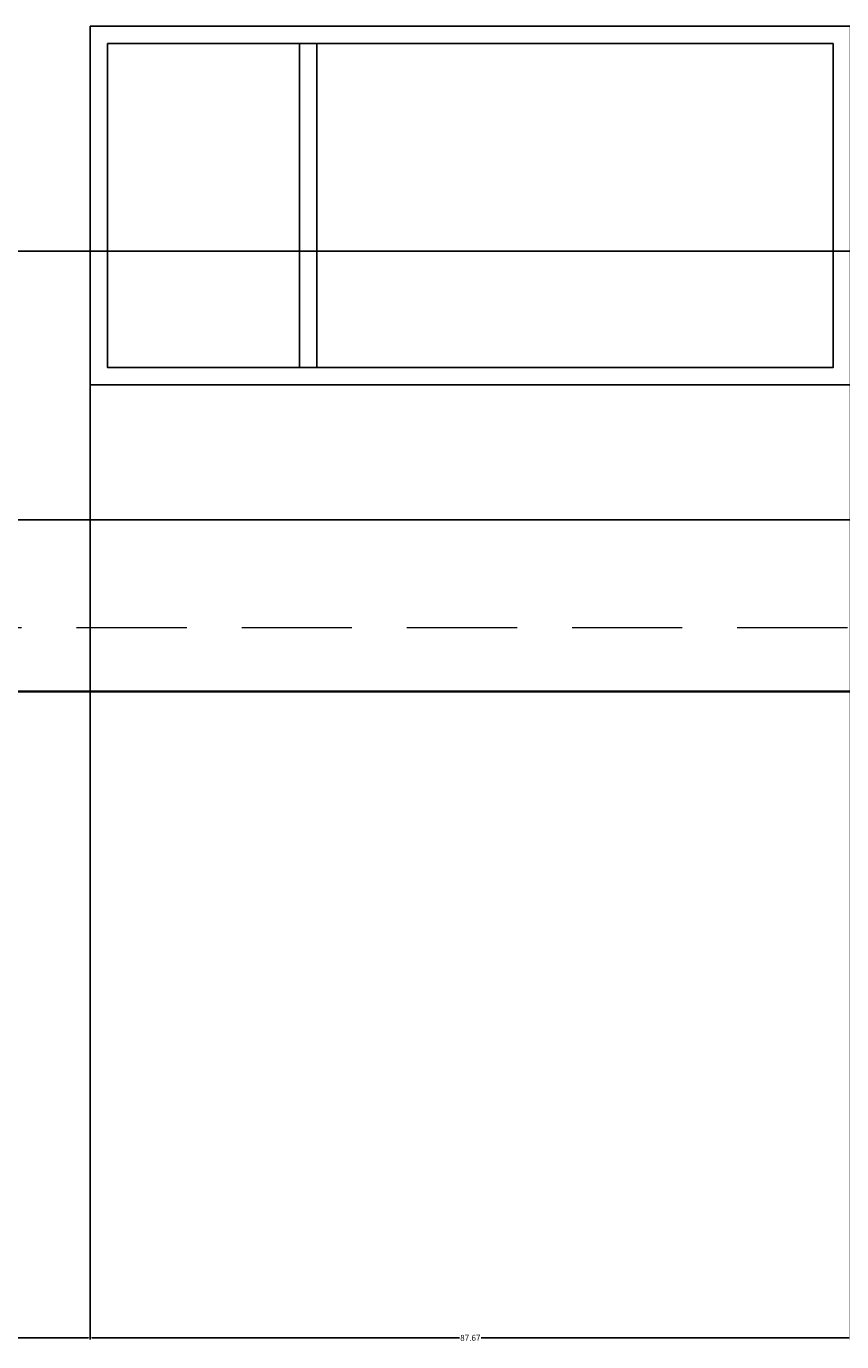
# Model space of a CAD drawing. Units: inches. Extents: x -145 to 510, y 5 to 386.
# Tile 17 of 25: x 346 to 440, y 5 to 157. Entities that reach past the tile are written whole.
import ezdxf

# ---------------------------------------------------------------- set-up
doc = ezdxf.new("R2010")
doc.units = ezdxf.units.IN
doc.header["$MEASUREMENT"] = 0
doc.linetypes.add('DASHED', pattern=[19.05, 12.7, -6.35])
for name, color, linetype, lineweight in [('A-ANNO-DIMS', 2, 'Continuous', 18), ('A-ELEV', 7, 'Continuous', 35), ('A-ELEV-HIDN', 8, 'DASHED', 18), ('A-GLAZ', 4, 'Continuous', 25)]:
    doc.layers.add(name, color=color, linetype=linetype, lineweight=lineweight)
doc.styles.get("Standard").update_dxf_attribs({"font": 'arial.ttf'})
doc.dimstyles.get("Standard").update_dxf_attribs({"dimtxt": 0.6875, "dimasz": 0.18, "dimexe": 0.18, "dimexo": 0.0625, "dimgap": 0.09, "dimtad": 0, "dimtih": 1, "dimtoh": 1, "dimdec": 4, "dimzin": 0, "dimdsep": 46, "dimlunit": 4, "dimtxsty": 'Standard', "dimcen": 0.09, "dimadec": 0, "dimazin": 0, "dimtfac": 1, "dimtdec": 4, "dimtofl": 0, "dimtmove": 0, "dimatfit": 3, "dimfxl": 1, "dimtolj": 1, "dimtzin": 0, "dimarcsym": 0})

# ---------------------------------------------------------------- blocks, each defined once
blk = doc.blocks.new('*D11')
at = {"layer": 'A-ANNO-DIMS', "color": 0, "lineweight": -2, "transparency": 16777216}
for p, q in [((353.23, 115.19), (353.23, 5.19)), ((315.55, 85.2), (315.55, 5.19)), ((315.73, 5.37), (333.14, 5.37)), ((353.05, 5.37), (335.64, 5.37))]:
    blk.add_line(p, q, dxfattribs=at)
at = {"layer": 'A-ANNO-DIMS', "color": 0, "transparency": 16777216}
for points in [[(315.73, 5.4), (315.73, 5.34), (315.55, 5.37)], [(353.05, 5.4), (353.05, 5.34), (353.23, 5.37)]]:
    blk.add_solid(points, dxfattribs=at)
at = {"layer": 'Defpoints', "color": 0, "transparency": 16777216}
for p in [(353.23, 115.26), (315.55, 85.26), (353.23, 5.37)]:
    blk.add_point(p, dxfattribs=at)
at = {"layer": 'A-ANNO-DIMS', "color": 0, "transparency": 16777216, "insert": (334.39, 5.37), "char_height": 0.688, "attachment_point": 5}
blk.add_mtext('\\A1;37.68', dxfattribs=at)
blk = doc.blocks.new('*D12')
at = {"layer": 'A-ANNO-DIMS', "color": 0, "lineweight": -2, "transparency": 16777216}
for p, q in [((353.23, 115.19), (353.23, 5.19)), ((440.9, 115.19), (440.9, 5.19)), ((353.41, 5.37), (395.82, 5.37)), ((440.72, 5.37), (398.32, 5.37))]:
    blk.add_line(p, q, dxfattribs=at)
at = {"layer": 'A-ANNO-DIMS', "color": 0, "transparency": 16777216}
for points in [[(353.41, 5.4), (353.41, 5.34), (353.23, 5.37)], [(440.72, 5.4), (440.72, 5.34), (440.9, 5.37)]]:
    blk.add_solid(points, dxfattribs=at)
at = {"layer": 'Defpoints', "color": 0, "transparency": 16777216}
for p in [(353.23, 115.26), (440.9, 115.26), (440.9, 5.37)]:
    blk.add_point(p, dxfattribs=at)
at = {"layer": 'A-ANNO-DIMS', "color": 0, "transparency": 16777216, "insert": (397.07, 5.37), "char_height": 0.688, "attachment_point": 5}
blk.add_mtext('\\A1;87.67', dxfattribs=at)
blk = doc.blocks.new('*D19')
at = {"layer": 'A-ANNO-DIMS', "color": 0, "lineweight": -2, "transparency": 16777216}
for p, q in [((478.76, 355.89), (-144.05, 355.89)), ((-143.87, 355.71), (-143.87, 218.33)), ((-143.87, 80.07), (-143.87, 217.45)), ((-114.04, 79.89), (-144.05, 79.89))]:
    blk.add_line(p, q, dxfattribs=at)
at = {"layer": 'A-ANNO-DIMS', "color": 0, "transparency": 16777216}
for points in [[(-143.9, 355.71), (-143.84, 355.71), (-143.87, 355.89)], [(-143.9, 80.07), (-143.84, 80.07), (-143.87, 79.89)]]:
    blk.add_solid(points, dxfattribs=at)
at = {"layer": 'Defpoints', "color": 0, "transparency": 16777216}
for p in [(-143.87, 355.89), (478.83, 355.89), (-113.97, 79.89)]:
    blk.add_point(p, dxfattribs=at)
at = {"layer": 'A-ANNO-DIMS', "color": 0, "transparency": 16777216, "insert": (-143.87, 217.89), "char_height": 0.688, "attachment_point": 5}
blk.add_mtext('\\A1;276', dxfattribs=at)
blk = doc.blocks.new('*D58')
at = {"layer": 'A-ANNO-DIMS', "color": 0, "lineweight": -2, "transparency": 16777216}
for p, q in [((265.82, 130.67), (508.91, 130.67)), ((508.73, 130.49), (508.73, 115.63)), ((508.73, 99.89), (508.73, 114.75)), ((265.82, 99.71), (508.91, 99.71))]:
    blk.add_line(p, q, dxfattribs=at)
at = {"layer": 'A-ANNO-DIMS', "color": 0, "transparency": 16777216}
for points in [[(508.7, 130.49), (508.76, 130.49), (508.73, 130.67)], [(508.7, 99.89), (508.76, 99.89), (508.73, 99.71)]]:
    blk.add_solid(points, dxfattribs=at)
at = {"layer": 'Defpoints', "color": 0, "transparency": 16777216}
for p in [(265.76, 130.67), (508.73, 130.67), (265.76, 99.71)]:
    blk.add_point(p, dxfattribs=at)
at = {"layer": 'A-ANNO-DIMS', "color": 0, "transparency": 16777216, "insert": (508.73, 115.19), "char_height": 0.688, "attachment_point": 5}
blk.add_mtext('\\A1;30.96', dxfattribs=at)

msp = doc.modelspace()

# ---------------------------------------------------------------- linework, layer by layer
at = {"layer": 'A-ELEV'}
for p in [(54.0014, 79.8905), (474.4893, 79.8905)]:
    msp.add_line(p, (392.4492, 79.8905), dxfattribs=at)
at = {"layer": 'A-ELEV-HIDN'}
msp.add_line((313.5545, 87.2638), (474.4893, 87.2638), dxfattribs=at)
at = {"layer": 'A-GLAZ'}
for p, q in [((377.3653, 154.6093), (377.3653, 117.2574)), ((379.3653, 154.6093), (379.3653, 117.2574))]:
    msp.add_line(p, q, dxfattribs=at)
for points in [[(353.234, 156.6093), (440.9009, 156.6093), (440.9009, 115.2574), (353.234, 115.2574)], [(355.234, 154.6093), (438.9009, 154.6093), (438.9009, 117.2574), (355.234, 117.2574)]]:
    msp.add_lwpolyline(points, close=True, dxfattribs=at)

# ---------------------------------------------------------------- dimensions: what is measured, and where the dimension line sits
at = {"layer": 'A-ANNO-DIMS'}
for base, p1, p2, override, picture, middle in [((-143.8737, 355.8905), (-113.9737, 79.8905), (478.8263, 355.8905), {"dimdec": 0, "dimlfac": 1, "dimrnd": 0, "dimzin": 0, "dimdsep": 46, "dimlunit": 2}, '*D19', (-143.8737, 217.8905)), ((508.7263, 130.6707), (265.7612, 99.7118), (265.7612, 130.6707), {"dimdec": 2, "dimlfac": 1, "dimrnd": 0, "dimzin": 0, "dimdsep": 46, "dimlunit": 2}, '*D58', (508.7263, 115.1912))]:
    dim = msp.add_linear_dim(base=base, p1=p1, p2=p2, angle=90, dimstyle='Standard', override=override, dxfattribs=at)
    dim.commit()
    dim.dimension.update_dxf_attribs({"geometry": picture, "text_midpoint": middle})
for base, p1, p2, picture, middle in [((353.234, 5.3738), (315.5545, 85.2638), (353.234, 115.2574), '*D11', (334.3942, 5.3738)), ((440.9009, 5.3738), (353.234, 115.2574), (440.9009, 115.2574), '*D12', (397.0675, 5.3738))]:
    dim = msp.add_linear_dim(base=base, p1=p1, p2=p2, dimstyle='Standard', override={"dimdec": 2, "dimlfac": 1, "dimrnd": 0, "dimzin": 0, "dimdsep": 46, "dimlunit": 2}, dxfattribs=at)
    dim.commit()
    dim.dimension.update_dxf_attribs({"geometry": picture, "text_midpoint": middle})

doc.saveas('drawing.dxf')
